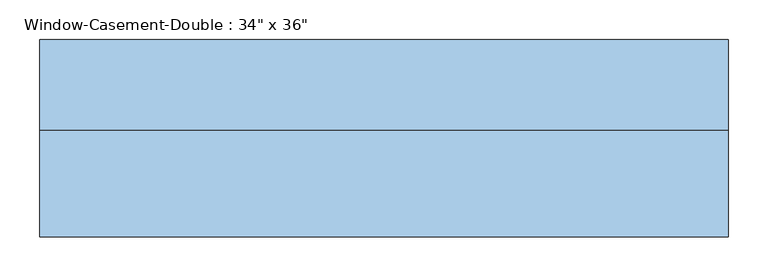
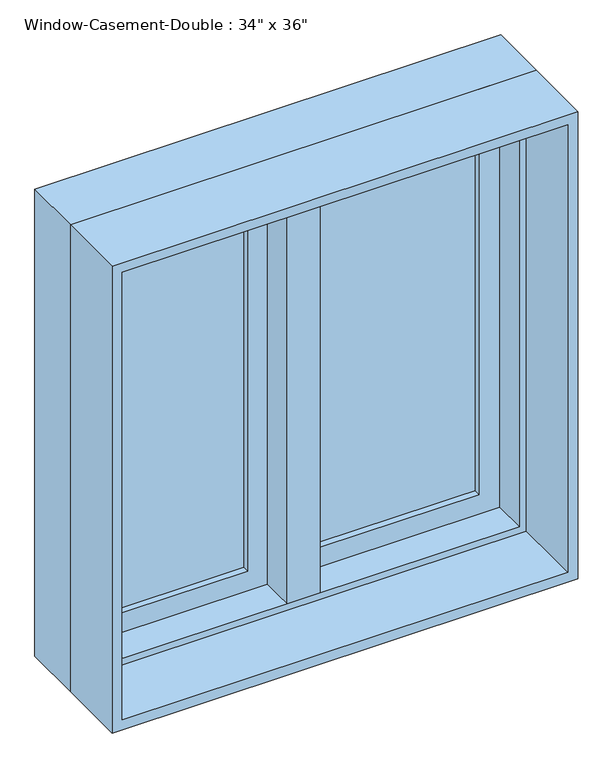
"""IFC4 building model written with IfcOpenShell, lengths in millimetres: window geometry."""

from ifc_helpers import new_model, si_unit, frame, origin, place, context, project, spatial, polyline, outline, extrude, faceted_brep, source, transform, mapped, element, save


def window_339605e1(model_context):
    return source(origin(), model_context, "Body", "SolidModel", [
        faceted_brep([(9.525, 133.35, 1816.1), (-9.525, 133.35, 1816.1), (-9.525, 82.55, 1816.1), (9.525, 82.55, 1816.1), (9.525, 133.35, 927.1), (9.525, 82.55, 927.1), (-9.525, 82.55, 927.1), (-9.525, 133.35, 927.1), (-9.525, 82.55, 946.15), (-9.525, 82.55, 1797.05), (-30.1625, 82.55, 946.15), (-30.1625, 82.55, 1797.05), (-30.1625, 19.05, 946.15), (-30.1625, 19.05, 1797.05), (30.1625, 19.05, 946.15), (30.1625, 19.05, 1797.05), (30.1625, 82.55, 946.15), (30.1625, 82.55, 1797.05), (9.525, 82.55, 946.15), (9.525, 82.55, 1797.05)], [[[0, 1, 2, 3]], [[4, 5, 6, 7]], [[1, 0, 4, 7]], [[2, 1, 7, 6, 8, 9]], [[9, 8, 10, 11]], [[11, 10, 12, 13]], [[13, 12, 14, 15]], [[15, 14, 16, 17]], [[17, 16, 18, 19]], [[0, 3, 19, 18, 5, 4]], [[18, 8, 6, 5]], [[9, 19, 3, 2]], [[8, 18, 16, 14, 12, 10]], [[19, 9, 11, 13, 15, 17]]]),
        extrude(outline(polyline([(-66.675, 114.3), (-66.675, 107.95), (-361.95, 107.95), (-361.95, 114.3), (-66.675, 114.3)])), frame((0.0, 0.0, 984.25), z_axis=(0.0, 0.0, 1.0), x_axis=(1.0, 0.0, 0.0)), (0.0, 0.0, 1.0), 774.7),
        extrude(outline(polyline([(-361.95, 95.25), (-361.95, 101.6), (-66.675, 101.6), (-66.675, 95.25), (-361.95, 95.25)])), frame((0.0, 0.0, 984.25), z_axis=(0.0, 0.0, 1.0), x_axis=(1.0, 0.0, 0.0)), (0.0, 0.0, 1.0), 774.7),
        extrude(outline(polyline([(361.95, 114.3), (361.95, 107.95), (66.675, 107.95), (66.675, 114.3), (361.95, 114.3)])), frame((0.0, 0.0, 984.25), z_axis=(0.0, 0.0, 1.0), x_axis=(1.0, 0.0, 0.0)), (0.0, 0.0, 1.0), 774.7),
        extrude(outline(polyline([(66.675, 95.25), (66.675, 101.6), (361.95, 101.6), (361.95, 95.25), (66.675, 95.25)])), frame((0.0, 0.0, 984.25), z_axis=(0.0, 0.0, 1.0), x_axis=(1.0, 0.0, 0.0)), (0.0, 0.0, 1.0), 774.7),
        extrude(outline(polyline([(1816.1, -419.1), (927.1, -419.1), (927.1, -9.525), (1816.1, -9.525), (1816.1, -419.1)]), holes=[polyline([(1758.95, -66.675), (984.25, -66.675), (984.25, -361.95), (1758.95, -361.95), (1758.95, -66.675)])]), frame((0.0, 82.55, 0.0), z_axis=(0.0, 1.0, 0.0), x_axis=(0.0, 0.0, 1.0)), (0.0, 0.0, 1.0), 44.45),
        extrude(outline(polyline([(927.1, 419.1), (1816.1, 419.1), (1816.1, 9.525), (927.1, 9.525), (927.1, 419.1)]), holes=[polyline([(984.25, 66.675), (1758.95, 66.675), (1758.95, 361.95), (984.25, 361.95), (984.25, 66.675)])]), frame((0.0, 82.55, 0.0), z_axis=(0.0, 1.0, 0.0), x_axis=(0.0, 0.0, 1.0)), (0.0, 0.0, 1.0), 44.45),
        extrude(outline(polyline([(1828.8, -431.8), (914.4, -431.8), (914.4, 431.8), (1828.8, 431.8), (1828.8, -431.8)]), holes=[polyline([(1809.75, 412.75), (933.45, 412.75), (933.45, -412.75), (1809.75, -412.75), (1809.75, 412.75)])]), frame((0.0, -114.3, 0.0), z_axis=(0.0, 1.0, 0.0), x_axis=(0.0, 0.0, 1.0)), (0.0, 0.0, 1.0), 133.35),
        faceted_brep([(400.05, 82.55, 1797.05), (400.05, 19.05, 1797.05), (-400.05, 19.05, 1797.05), (-400.05, 82.55, 1797.05), (419.1, 133.35, 1816.1), (419.1, 82.55, 1816.1), (-419.1, 82.55, 1816.1), (-419.1, 133.35, 1816.1), (431.8, 19.05, 1828.8), (431.8, 133.35, 1828.8), (-431.8, 133.35, 1828.8), (-431.8, 19.05, 1828.8), (-400.05, 19.05, 946.15), (-400.05, 82.55, 946.15), (-419.1, 82.55, 927.1), (-419.1, 133.35, 927.1), (-431.8, 133.35, 914.4), (-431.8, 19.05, 914.4), (400.05, 19.05, 946.15), (400.05, 82.55, 946.15), (419.1, 82.55, 927.1), (419.1, 133.35, 927.1), (431.8, 133.35, 914.4), (431.8, 19.05, 914.4)], [[[0, 1, 2, 3]], [[4, 5, 6, 7]], [[8, 9, 10, 11]], [[3, 2, 12, 13]], [[7, 6, 14, 15]], [[11, 10, 16, 17]], [[13, 12, 18, 19]], [[15, 14, 20, 21]], [[17, 16, 22, 23]], [[11, 17, 23, 8], [1, 18, 12, 2]], [[19, 18, 1, 0]], [[5, 20, 14, 6], [3, 13, 19, 0]], [[21, 20, 5, 4]], [[23, 22, 9, 8]], [[9, 22, 16, 10], [7, 15, 21, 4]]]),
    ])


if __name__ == "__main__":
    model = new_model("IFC4")
    model_context = context("Model", 3, world=origin())
    ifc_project = project(units=[si_unit("LENGTHUNIT", "METRE", prefix="MILLI")], contexts=[model_context])
    site = spatial("IfcSite", under=ifc_project)
    building = spatial("IfcBuilding", under=site)
    placement = place(None, origin())
    window_shape = window_339605e1(model_context)
    element("IfcWindow", 1, ObjectType="Window-Casement-Double : 34\" x 36\"", at=placement, inside=building, context=model_context, shape_type="MappedRepresentation", body=[
        mapped(window_shape, transform((0.0, 0.0, 0.0), x_axis=(1.0, 0.0, 0.0), y_axis=(0.0, 1.0, 0.0), z_axis=(0.0, 0.0, 1.0))),
    ])
    save(model, "model.ifc")

# Revit data of these elements
# Type "Window-Casement-Double : 34\" x 36\""
#   Type Mark = "14"
#   Fire Rating = "0.5h"
#   Assembly Code = "B2020100"
#   Analytic Construction = "Double glazing - domestic"
#   Frame Extension [instance default] = 0' - 0 1/4"
#   Window Inset [instance default] = 0' - 0"
#   Wall Thickness [instance default] = 0' - 6"
#   Interior Wall Closure [instance default] = 0' - 2 1/4"
#   Half Width = 1' - 5"
#   Visual Light Transmittance = 0.81
#   Thermal Resistance (R) = 1.8146 (h·ft²·°F)/BTU
#   Solar Heat Gain Coefficient = 0.76
#   Rough Width = 2' - 10 1/2"
#   Rough Height = 3' - 0 1/2"
#   Height = 3' - 0"
#   Heat Transfer Coefficient (U) = 0.5511 BTU/(h·ft²·°F)
#   Exterior Wall Closure [instance default] = 0' - 1 1/4"
#   Extension Jamb [instance default] = 0' - 2 1/4"
#   Default Sill Height = 3' - 0"
#   Width = 2' - 10"
#   Define Thermal Properties by = 0
#   Muntin Visibility = yes
#   Interior Trim Visibility [instance default] = yes
#   Exterior Trim Visibility [instance default] = yes
#   Extension Jamb Visibility [instance default] = yes
#   Interior Trim Material = Wood - Stained
#   Muntin Pattern = Muntin Pattern_2x2 : Muntin Pattern_2x2
#   Interior Trim = Trim-Window-Interior-Flat : Picture Frame
#   Interior Frame Material = Wood - Stained
#   Glass Panel Material = Glass
#   Exterior Trim Material = Clad - White
#   Exterior Trim = Trim-Window-Exterior-Flat : with Sill
#   Exterior Frame Material = Clad - White
#   Wall Closure = (empty or 0)
# Element 1 (IfcWindow, "Window-Casement-Double : 34\" x 36\"")
#   Wall Thickness = 0' - 9"
#   Extension Jamb = 0' - 5 1/4"
#   Materials on its faces: "Wood - Stained", "Glass", "Clad - White"
# Materials
#   "Wood - Stained": class "Wood", colour RGB 224 178 126, transparency 0, Cost = 0
#   "Glass": class "Glass", colour RGB 0 128 192, transparency 0.75, Description = "Soda Lime Glass", Cost = 0
#   "Clad - White": class "Wood", colour RGB 242 242 238, transparency 0, Cost = 0
